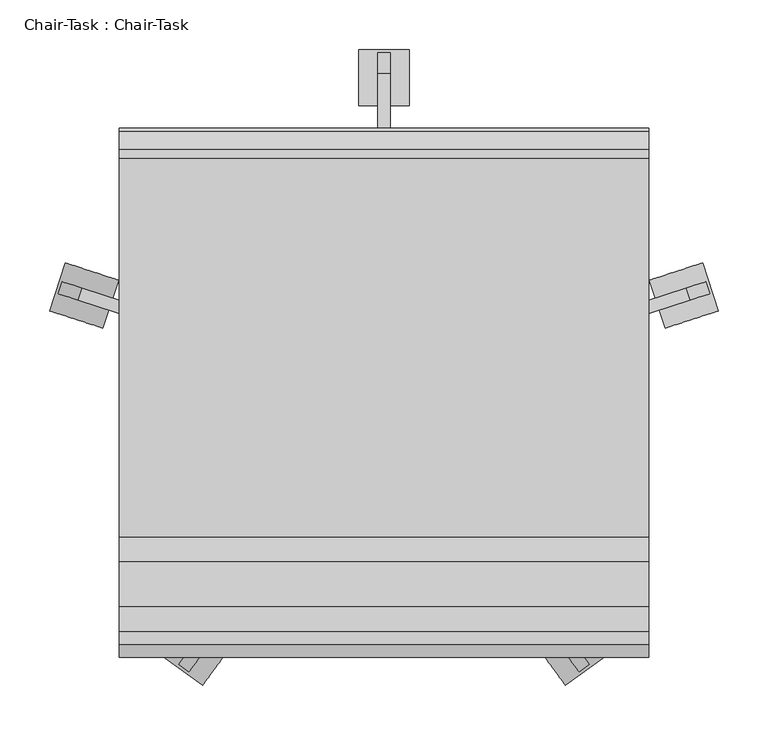
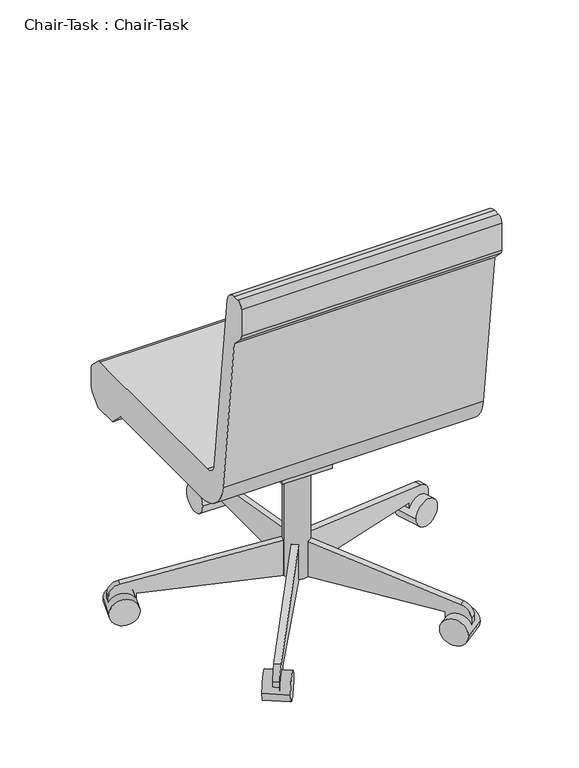
"""IFC4 building model written with IfcOpenShell, lengths in millimetres: furniture geometry, Chair-Task : Chair-Task."""

from ifc_helpers import new_model, si_unit, point, frame, frame_2d, origin, place, context, project, spatial, polyline, circle_curve, trimmed, segment, composite_curve, outline, extrude, source, transform, mapped, element, save


def chair_task_chair_task_b7f3823b(model_context):
    return source(origin(), model_context, "Body", "SweptSolid", [
        extrude(outline(composite_curve([segment(trimmed(circle_curve(frame_2d((140.9908197, 18.9459016)), 25.4), [point((115.5908197, 18.9459016))], [point((166.3908197, 18.9459016))], False, "CARTESIAN"), True, "CONTINUOUS"), segment(trimmed(circle_curve(frame_2d((140.9908197, 18.9459016)), 25.4), [point((166.3908197, 18.9459016))], [point((115.5908197, 18.9459016))], False, "CARTESIAN"), True, "CONTINUOUS")], self_intersect=False)), frame((0.0, 0.0, 53.5835944), z_axis=(0.0, 0.0, 1.0), x_axis=(1.0, 0.0, 0.0)), (0.0, 0.0, 1.0), 330.5914056),
        extrude(outline(composite_curve([segment(trimmed(circle_curve(frame_2d((0.0, -28.2002727)), 28.2002727), [point((0.0, -56.4005455))], [point((0.0, 0.0))], False, "CARTESIAN"), True, "CONTINUOUS"), segment(trimmed(circle_curve(frame_2d((0.0, -28.2002727)), 28.2002727), [point((0.0, 0.0))], [point((0.0, -56.4005455))], False, "CARTESIAN"), True, "CONTINUOUS")], self_intersect=False)), frame((477.6203484, 101.6163254, 28.1835944), z_axis=(-0.3090169943749423, 0.9510565162951553, 0.0), x_axis=(0.0, 0.0, 1.0)), (0.0, 0.0, 1.0), 50.8),
        extrude(outline(composite_curve([segment(polyline([(-25.4, 0.0), (0.0, 0.0), (0.0, -50.8), (-24.303053, -50.8)]), True, "CONTINUOUS"), segment(trimmed(circle_curve(frame_2d((-24.303053, -25.4)), 25.4), [point((-24.303053, -50.8))], [point((-49.3171699, -29.8106637))], False, "CARTESIAN"), True, "CONTINUOUS"), segment(polyline([(-49.3171699, -29.8106637), (-101.6, 266.7), (-101.6, 292.1), (-25.4, 292.1), (-25.4, 0.0)]), True, "CONTINUOUS")], self_intersect=False)), frame((420.756686, 103.1705568, 28.1835944), z_axis=(-0.3090169943749423, 0.9510565162951553, 0.0), x_axis=(0.0, 0.0, -1.0)), (0.0, 0.0, 1.0), 12.7),
        extrude(outline(composite_curve([segment(trimmed(circle_curve(frame_2d((0.0, -28.2002727)), 28.2002727), [point((0.0, -56.4005455))], [point((0.0, 0.0))], False, "CARTESIAN"), True, "CONTINUOUS"), segment(trimmed(circle_curve(frame_2d((0.0, -28.2002727)), 28.2002727), [point((0.0, 0.0))], [point((0.0, -56.4005455))], False, "CARTESIAN"), True, "CONTINUOUS")], self_intersect=False)), frame((323.63931, -275.6612394, 28.1835944), z_axis=(0.8090169943749499, 0.5877852522924699, 0.0), x_axis=(0.0, 0.0, 1.0)), (0.0, 0.0, 1.0), 50.8),
        extrude(outline(composite_curve([segment(polyline([(-25.4, 0.0), (0.0, 0.0), (0.0, -50.8), (-24.303053, -50.8)]), True, "CONTINUOUS"), segment(trimmed(circle_curve(frame_2d((-24.303053, -25.3999999)), 25.4), [point((-24.303053, -50.8))], [point((-49.3171699, -29.8106636))], False, "CARTESIAN"), True, "CONTINUOUS"), segment(polyline([(-49.3171699, -29.8106636), (-101.6, 266.7), (-101.6, 292.1), (-25.4, 292.1), (-25.4, 0.0)]), True, "CONTINUOUS")], self_intersect=False)), frame((307.545634, -221.1003988, 28.1835944), z_axis=(0.8090169943749499, 0.5877852522924699, 0.0), x_axis=(0.0, 0.0, -1.0)), (0.0, 0.0, 1.0), 12.7),
        extrude(outline(composite_curve([segment(trimmed(circle_curve(frame_2d((0.0, -28.2002727)), 28.2002727), [point((0.0, -56.4005455))], [point((0.0, 0.0))], False, "CARTESIAN"), True, "CONTINUOUS"), segment(trimmed(circle_curve(frame_2d((0.0, -28.2002727)), 28.2002727), [point((0.0, 0.0))], [point((0.0, -56.4005455))], False, "CARTESIAN"), True, "CONTINUOUS")], self_intersect=False)), frame((-41.6576707, -275.6612394, 28.1835944), z_axis=(-0.8090169943749458, 0.5877852522924754, 0.0), x_axis=(0.0, 0.0, -1.0)), (0.0, 0.0, 1.0), 50.8),
        extrude(outline(composite_curve([segment(polyline([(25.4, 0.0), (25.4, 292.1), (101.6, 292.1), (101.6, 266.7), (49.3171699, -29.8106637)]), True, "CONTINUOUS"), segment(trimmed(circle_curve(frame_2d((24.303053, -25.3999999)), 25.4), [point((49.3171699, -29.8106637))], [point((24.303053, -50.8))], False, "CARTESIAN"), True, "CONTINUOUS"), segment(polyline([(24.303053, -50.8), (0.0, -50.8), (0.0, 0.0), (25.4, 0.0)]), True, "CONTINUOUS")], self_intersect=False)), frame((-25.5639946, -221.1003988, 28.1835944), z_axis=(-0.8090169943749459, 0.5877852522924754, 0.0), x_axis=(0.0, 0.0, 1.0)), (0.0, 0.0, 1.0), 12.7),
        extrude(outline(composite_curve([segment(trimmed(circle_curve(frame_2d((0.0, -28.2002727)), 28.2002727), [point((0.0, -56.4005454))], [point((0.0, 0.0))], False, "CARTESIAN"), True, "CONTINUOUS"), segment(trimmed(circle_curve(frame_2d((0.0, -28.2002727)), 28.2002727), [point((0.0, 0.0))], [point((0.0, -56.4005454))], False, "CARTESIAN"), True, "CONTINUOUS")], self_intersect=False)), frame((-195.638709, 101.6163254, 28.1835944), z_axis=(0.3090169943749487, 0.9510565162951532, 0.0), x_axis=(0.0, 0.0, -1.0)), (0.0, 0.0, 1.0), 50.8),
        extrude(outline(composite_curve([segment(polyline([(25.4, 0.0), (25.4, 292.1000001), (101.6, 292.1000001), (101.6, 266.7), (49.3171699, -29.8106636)]), True, "CONTINUOUS"), segment(trimmed(circle_curve(frame_2d((24.303053, -25.4)), 25.4), [point((49.3171699, -29.8106636))], [point((24.303053, -50.8))], False, "CARTESIAN"), True, "CONTINUOUS"), segment(polyline([(24.303053, -50.8), (0.0, -50.8), (0.0, 0.0), (25.4, 0.0)]), True, "CONTINUOUS")], self_intersect=False)), frame((-138.7750467, 103.1705568, 28.1835944), z_axis=(0.3090169943749487, 0.9510565162951532, 0.0), x_axis=(0.0, 0.0, 1.0)), (0.0, 0.0, 1.0), 12.7),
        extrude(outline(composite_curve([segment(trimmed(circle_curve(frame_2d((336.4459016, 28.1835944)), 28.2002727), [point((308.2456289, 28.1835944))], [point((364.6461744, 28.1835944))], False, "CARTESIAN"), True, "CONTINUOUS"), segment(trimmed(circle_curve(frame_2d((336.4459016, 28.1835944)), 28.2002727), [point((364.6461744, 28.1835944))], [point((308.2456289, 28.1835944))], False, "CARTESIAN"), True, "CONTINUOUS")], self_intersect=False)), frame((115.5908197, 0.0, 0.0), z_axis=(1.0, 0.0, 0.0), x_axis=(0.0, 1.0, 0.0)), (0.0, 0.0, 1.0), 50.8),
        extrude(outline(composite_curve([segment(polyline([(311.0459016, 53.5835944), (18.9459016, 53.5835944), (18.9459016, 129.7835944), (44.3459016, 129.7835944), (340.8565654, 77.5007643)]), True, "CONTINUOUS"), segment(trimmed(circle_curve(frame_2d((336.4459016, 52.4866474)), 25.4), [point((340.8565654, 77.5007643))], [point((361.8459016, 52.4866474))], False, "CARTESIAN"), True, "CONTINUOUS"), segment(polyline([(361.8459016, 52.4866474), (361.8459016, 28.1835944), (311.0459016, 28.1835944), (311.0459016, 53.5835944)]), True, "CONTINUOUS")], self_intersect=False)), frame((134.6408197, 0.0, 0.0), z_axis=(1.0, 0.0, 0.0), x_axis=(0.0, 1.0, 0.0)), (0.0, 0.0, 1.0), 12.7),
        extrude(outline(polyline([(69.7459016, 383.7835944), (69.7459016, 371.0835944), (18.9459016, 283.0954134), (-19.1540984, 283.0954134), (-19.1540984, 383.7835944), (69.7459016, 383.7835944)])), frame((90.1908197, 0.0, 0.0), z_axis=(1.0, 0.0, 0.0), x_axis=(0.0, 1.0, 0.0)), (0.0, 0.0, 1.0), 101.6),
        extrude(outline(composite_curve([segment(polyline([(-126.2050455, 457.2), (255.0102301, 457.2)]), True, "CONTINUOUS"), segment(trimmed(circle_curve(frame_2d((255.0102301, 444.5)), 12.7), [point((255.0102301, 457.2))], [point((263.9604301, 453.510212))], False, "CARTESIAN"), True, "CONTINUOUS"), segment(polyline([(263.9604301, 453.510212), (281.8961016, 435.6939999)]), True, "CONTINUOUS"), segment(trimmed(circle_curve(frame_2d((272.9459016, 426.6837879)), 12.7), [point((281.8961016, 435.6939999))], [point((285.6459016, 426.6837879))], False, "CARTESIAN"), True, "CONTINUOUS"), segment(polyline([(285.6459016, 426.6837879), (285.6459016, 391.6405184)]), True, "CONTINUOUS"), segment(trimmed(circle_curve(frame_2d((260.2459016, 391.6405184)), 25.4), [point((285.6459016, 391.6405184))], [point((278.2663256, 373.7401184))], False, "CARTESIAN"), True, "CONTINUOUS"), segment(polyline([(278.2663256, 373.7401184), (260.2470284, 355.6), (209.4470284, 355.6), (181.0744602, 383.7835944), (-107.1089978, 383.7835944)]), True, "CONTINUOUS"), segment(trimmed(circle_curve(frame_2d((-107.1089978, 459.9835944)), 76.2), [point((-107.1089978, 383.7835944))], [point((-182.7870738, 451.0802913))], False, "CARTESIAN"), True, "CONTINUOUS"), segment(polyline([(-182.7870738, 451.0802913), (-222.3540984, 787.4), (-244.0343545, 809.0802561)]), True, "CONTINUOUS"), segment(trimmed(circle_curve(frame_2d((-235.0540984, 818.0605122)), 12.7), [point((-244.0343545, 809.0802561))], [point((-247.7540984, 818.0605122))], False, "CARTESIAN"), True, "CONTINUOUS"), segment(polyline([(-247.7540984, 818.0605122), (-247.7540984, 876.3)]), True, "CONTINUOUS"), segment(trimmed(circle_curve(frame_2d((-235.0540984, 876.3)), 12.7), [point((-247.7540984, 876.3))], [point((-235.0540984, 889.0))], False, "CARTESIAN"), True, "CONTINUOUS"), segment(polyline([(-235.0540984, 889.0), (-222.1789239, 889.0)]), True, "CONTINUOUS"), segment(trimmed(circle_curve(frame_2d((-222.1789239, 863.6)), 25.4), [point((-222.1789239, 889.0))], [point((-196.9528985, 866.5677677))], False, "CARTESIAN"), True, "CONTINUOUS"), segment(polyline([(-196.9528985, 866.5677677), (-151.4310708, 479.6322323)]), True, "CONTINUOUS"), segment(trimmed(circle_curve(frame_2d((-126.2050455, 482.6)), 25.4), [point((-151.4310708, 479.6322323))], [point((-126.2050455, 457.2))], True, "CARTESIAN"), True, "CONTINUOUS")], self_intersect=False)), frame((-125.7091803, 0.0, 0.0), z_axis=(1.0, 0.0, 0.0), x_axis=(0.0, 1.0, 0.0)), (0.0, 0.0, 1.0), 533.4),
    ])


if __name__ == "__main__":
    model = new_model("IFC4")
    model_context = context("Model", 3, world=origin())
    ifc_project = project(units=[si_unit("LENGTHUNIT", "METRE", prefix="MILLI")], contexts=[model_context])
    site = spatial("IfcSite", under=ifc_project)
    building = spatial("IfcBuilding", under=site)
    placement = place(None, origin())
    chair_task_chair_task_shape = chair_task_chair_task_b7f3823b(model_context)
    element("IfcFurniture", 1, ObjectType="Chair-Task : Chair-Task", at=placement, inside=building, context=model_context, shape_type="MappedRepresentation", body=[
        mapped(chair_task_chair_task_shape, transform((0.0, 0.0, 0.0), x_axis=(1.0, 0.0, 0.0), y_axis=(0.0, 1.0, 0.0), z_axis=(0.0, 0.0, 1.0))),
    ])
    save(model, "model.ifc")

# Revit data of these elements
# Type "Chair-Task : Chair-Task"
#   Assembly Code = "E2020200"
#   Base Material = Plastic - Black
#   Caster Material = Plastic - Black
#   Seat/Back Material = Textile - Slate Blue
#   Default Elevation = 0
# Element 1 (IfcFurniture, "Chair-Task : Chair-Task")
#   Materials on its faces: "Plastic - Black", "Textile - Slate Blue"
# Materials
#   "Plastic - Black": colour RGB 0 0 0, transparency 0
#   "Textile - Slate Blue": colour RGB 98 102 118, transparency 0
